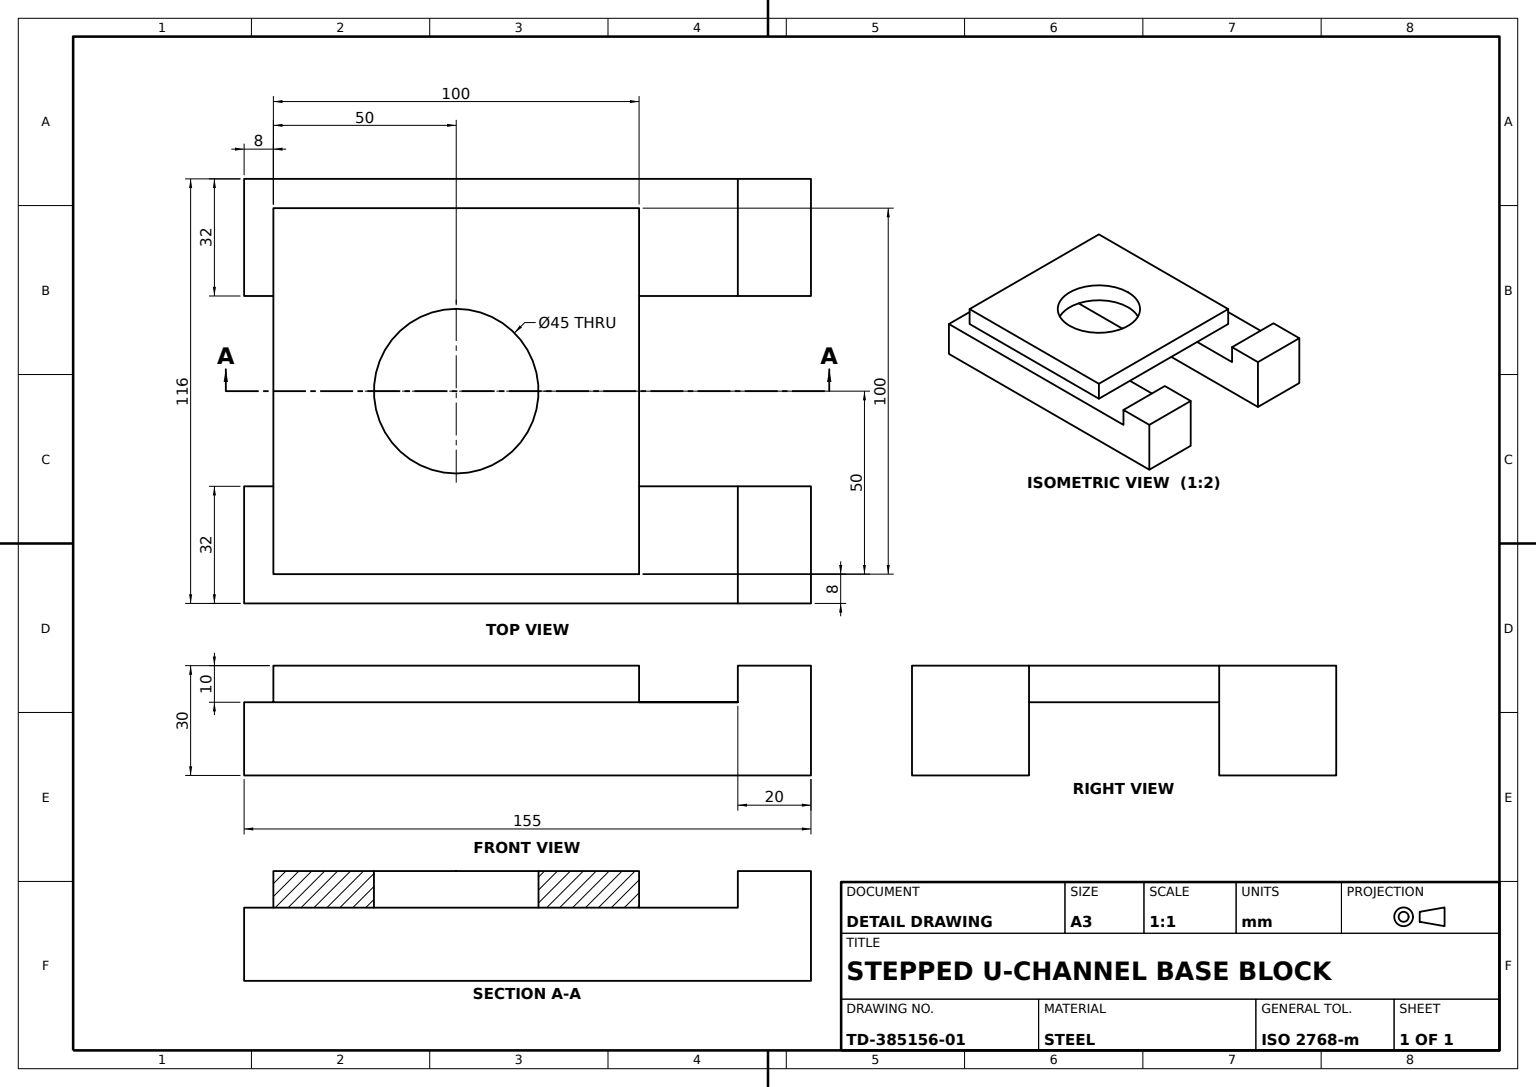
from build123d import *

# Parameters (mm, degrees)
BASE_PLATE_SKETCH_W              = 100
BASE_PLATE_SKETCH_H              = 100
BASE_PLATE_SKETCH_R              = 22.5
BASE_PLATE_100X100_BORE_45_DEPTH = 10
SIDE_RAILS_SKETCH_W              = 155
SIDE_RAILS_SKETCH_H              = 32
SIDE_RAILS_DEPTH                 = 20
END_BLOCKS_SKETCH_W              = 20
END_BLOCKS_SKETCH_H              = 32
END_BLOCKS_20X20_DEPTH           = 10


with BuildPart() as part:
    # Base Plate Sketch → Base Plate 100x100 Bore Ø45 (new body)
    with BuildSketch(Plane(origin=(0, 0, 0), x_dir=(1, 0, 0), z_dir=(0, 1, 0))):
        Rectangle(BASE_PLATE_SKETCH_W, BASE_PLATE_SKETCH_H)
        with Locations(Location((0, 0, 0), (0, 0, 270))):
            Circle(BASE_PLATE_SKETCH_R, mode=Mode.SUBTRACT)
    extrude(amount=BASE_PLATE_100X100_BORE_45_DEPTH)

    # Side Rails Sketch → Side Rails (add)
    with BuildSketch(Plane.XZ):
        with Locations((19.5, 42)):
            Rectangle(SIDE_RAILS_SKETCH_W, SIDE_RAILS_SKETCH_H)
        with Locations((19.5, -42)):
            Rectangle(SIDE_RAILS_SKETCH_W, SIDE_RAILS_SKETCH_H)
    extrude(amount=SIDE_RAILS_DEPTH)

    # End Blocks Sketch → End Blocks 20x20 (add)
    with BuildSketch(Plane(origin=(0, 0, 0), x_dir=(1, 0, 0), z_dir=(0, 1, 0))):
        with Locations((87, 42)):
            Rectangle(END_BLOCKS_SKETCH_W, END_BLOCKS_SKETCH_H)
        with Locations((87, -42)):
            Rectangle(END_BLOCKS_SKETCH_W, END_BLOCKS_SKETCH_H)
    extrude(amount=END_BLOCKS_20X20_DEPTH)


solid = part.part
